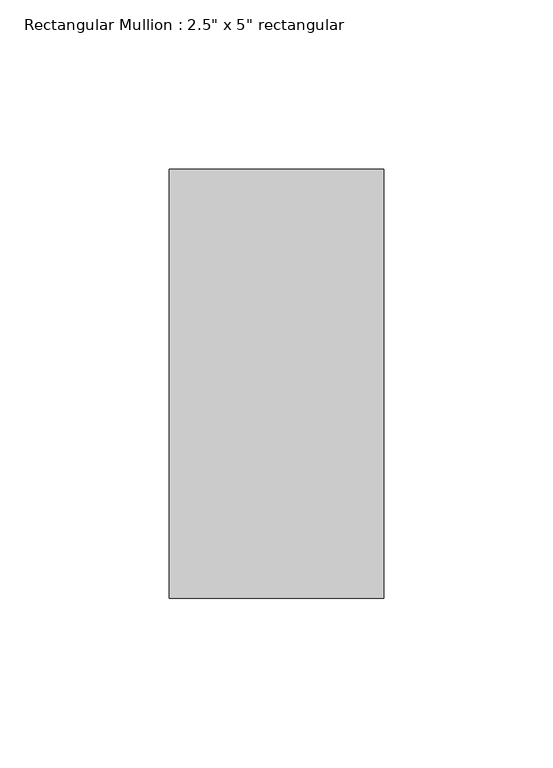
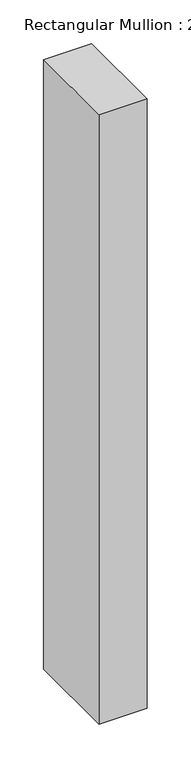
"""IFC4 building model written with IfcOpenShell, lengths in millimetres: member geometry."""

from ifc_helpers import new_model, si_unit, frame, origin, place, context, project, spatial, polyline, outline, extrude, source, transform, mapped, element, save


def member_95153237(model_context):
    return source(origin(), model_context, "Body", "SweptSolid", [
        extrude(outline(polyline([(31.75, 63.5), (31.75, -63.5), (-31.75, -63.5), (-31.75, 63.5), (31.75, 63.5)])), frame((0.0, 0.0, -850.8999998), z_axis=(0.0, 0.0, 1.0), x_axis=(1.0, 0.0, 0.0)), (0.0, 0.0, 1.0), 850.8999998),
    ])


if __name__ == "__main__":
    model = new_model("IFC4")
    model_context = context("Model", 3, world=origin())
    ifc_project = project(units=[si_unit("LENGTHUNIT", "METRE", prefix="MILLI")], contexts=[model_context])
    site = spatial("IfcSite", under=ifc_project)
    building = spatial("IfcBuilding", under=site)
    placement = place(None, origin())
    member_shape = member_95153237(model_context)
    element("IfcMember", 1, ObjectType="Rectangular Mullion : 2.5\" x 5\" rectangular", at=placement, inside=building, context=model_context, shape_type="MappedRepresentation", body=[
        mapped(member_shape, transform((0.0, 0.0, 0.0), x_axis=(1.0, 0.0, 0.0), y_axis=(0.0, 1.0, 0.0), z_axis=(0.0, 0.0, 1.0))),
    ])
    save(model, "model.ifc")

# Revit data of these elements
# Type "Rectangular Mullion : 2.5\" x 5\" rectangular"
#   built-in parameter 1007304 = 0.416667 (stored number, unit not read)
#   built-in parameter 1007301 = 0.104167 (stored number, unit not read)
#   built-in parameter 1007300 = 0.104167 (stored number, unit not read)
# Element 1 (IfcMember, "Rectangular Mullion : 2.5\" x 5\" rectangular")
#   Materials on its faces: "Aluminum"
# Materials
#   "Aluminum": class "Metal", colour RGB 247 247 247, transparency 0, Description = "Aluminum 6061", Cost = 0
